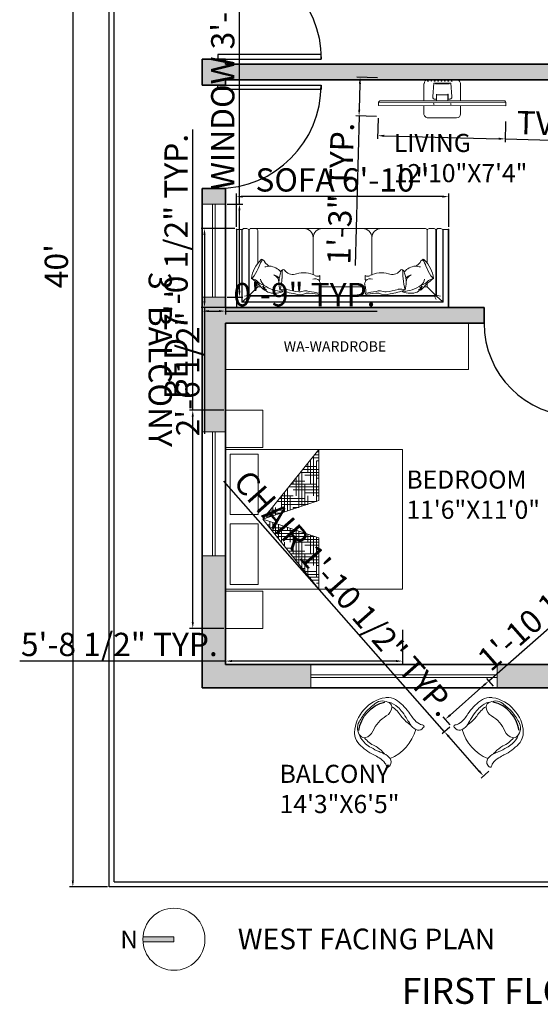
# Model space of a CAD drawing. Units: inches. Extents: x 2831 to 4250, y 1103 to 1797.
# Tile 1 of 15: x 3409 to 3610, y 1197 to 1578. Entities that reach past the tile are written whole.
import ezdxf

# ---------------------------------------------------------------- set-up
doc = ezdxf.new("R2010")
doc.units = ezdxf.units.IN
for name, color, linetype, lineweight in [('A-ANNO-DIMS', 2, 'Continuous', 18), ('A-ANNO-SYMB', 7, 'Continuous', 18), ('A-ANNO-TEXT', 7, 'Continuous', 18), ('A-ANNO-TITL', 7, 'Continuous', 25), ('A-AREA-IDEN', 7, 'Continuous', 18), ('A-DOOR', 4, 'Continuous', 25), ('A-EQPM', 8, 'Continuous', 18), ('A-FLOR-CASE', 9, 'Continuous', 18), ('A-WALL', 7, 'Continuous', 35), ('A-WALL-PATT', 252, 'Continuous', 13), ('C-PROP', 7, 'Continuous', 25), ('furn', 8, 'Continuous', 18), ('window', 130, 'Continuous', 18)]:
    doc.layers.add(name, color=color, linetype=linetype, lineweight=lineweight)
doc.layers.add('IFF-FURN-DETAIL', color=250, linetype='Continuous')
doc.styles.get("Standard").update_dxf_attribs({"font": 'arial.ttf'})
doc.dimstyles.new('ISO-25', dxfattribs={"dimtxt": 9, "dimasz": 2.5, "dimexe": 1.25, "dimexo": 0.625, "dimtad": 1, "dimdec": 1, "dimlunit": 3, "dimtxsty": 'Standard', "dimcen": 2.5, "dimadec": 0, "dimazin": 0, "dimtfac": 1, "dimtdec": 1, "dimtmove": 0, "dimatfit": 3, "dimfxl": 1, "dimarcsym": 0})

# ---------------------------------------------------------------- blocks, each defined once
blk = doc.blocks.new('*U2')
for p, q in [((0, 0), (0, -6)), ((40, 0), (40, -6))]:
    blk.add_line(p, q)
blk.add_lwpolyline([(0, 0), (0, 40), (1.75, 40), (1.75, 0)], close=True)
blk.add_arc((0, 0), 40, 0, 90)
blk = doc.blocks.new('*U3')
for p, q in [((0, 0), (0, -6)), ((36, 0), (36, -6))]:
    blk.add_line(p, q)
blk.add_lwpolyline([(0, 0), (0, 36), (1.75, 36), (1.75, 0)], close=True)
blk.add_arc((0, 0), 36, 0, 90)
blk = doc.blocks.new('*D6')
at = {"layer": 'A-ANNO-DIMS', "color": 0, "lineweight": -2, "transparency": 16777216}
for p, q in [((3442.6, 1722.51), (3427.96, 1722.51)), ((3429.21, 1720.01), (3429.21, 1245.01)), ((3442.6, 1242.51), (3427.96, 1242.51))]:
    blk.add_line(p, q, dxfattribs=at)
at = {"layer": 'A-ANNO-DIMS', "color": 0, "transparency": 16777216}
for points in [[(3428.79, 1720.01), (3429.62, 1720.01), (3429.21, 1722.51)], [(3428.79, 1245.01), (3429.62, 1245.01), (3429.21, 1242.51)]]:
    blk.add_solid(points, dxfattribs=at)
at = {"layer": 'Defpoints', "color": 0, "transparency": 16777216}
for p in [(3443.23, 1722.51), (3429.21, 1242.51), (3443.23, 1242.51)]:
    blk.add_point(p, dxfattribs=at)
at = {"layer": 'A-ANNO-DIMS', "color": 0, "transparency": 16777216, "insert": (3423.99, 1482.51), "char_height": 9, "attachment_point": 5, "rotation": 90}
blk.add_mtext("40'", dxfattribs=at)
blk = doc.blocks.new('COUCH6')
at = {"layer": 'furn'}
for p, q in [((-1.15, -0.846), (-1.15, 0)), ((-1.15, 0), (0, 0)), ((1.15, 0), (0, 0)), ((1.15, -0.846), (1.15, 0)), ((-1.145, -0.846), (-1.145, -0.005)), ((-1.145, -0.005), (0, -0.005)), ((-1.091, -0.845), (-1.091, -0.058)), ((-1.091, -0.058), (0, -0.058)), ((-1.086, -0.835), (-1.086, -0.063)), ((-1.086, -0.063), (0, -0.063)), ((-1.016, -0.124), (-1.086, -0.063)), ((-1.001, -0.114), (-1.014, -0.087)), ((1.145, -0.005), (0, -0.005)), ((1.091, -0.058), (0, -0.058)), ((1.086, -0.063), (0, -0.063)), ((1.001, -0.114), (1.014, -0.087)), ((1.016, -0.124), (1.086, -0.063)), ((1.086, -0.835), (1.086, -0.063)), ((1.091, -0.845), (1.091, -0.058)), ((1.145, -0.846), (1.145, -0.005)), ((-1.026, -0.131), (-1.061, -0.121)), ((-1.016, -0.835), (-1.016, -0.124)), ((-1.016, -0.124), (0, -0.124)), ((-1.011, -0.835), (-1.011, -0.129)), ((-1.011, -0.129), (0, -0.129)), ((-0.917, -0.223), (-1.011, -0.129)), ((-0.651, -0.171), (-0.652, -0.18)), ((1.016, -0.124), (0, -0.124)), ((1.011, -0.129), (0, -0.129)), ((0.651, -0.171), (0.652, -0.18)), ((0.917, -0.223), (1.011, -0.129)), ((1.011, -0.835), (1.011, -0.129)), ((1.016, -0.835), (1.016, -0.124)), ((1.026, -0.131), (1.061, -0.121)), ((-0.917, -0.223), (-0.884, -0.223)), ((-0.917, -0.259), (-0.917, -0.223)), ((-0.247, -0.223), (0, -0.223)), ((0.247, -0.223), (0, -0.223)), ((0.917, -0.223), (0.884, -0.223)), ((0.917, -0.259), (0.917, -0.223)), ((-0.665, -0.398), (-0.674, -0.359)), ((-0.651, -0.409), (-0.665, -0.398)), ((-0.318, -0.755), (-0.318, -0.351)), ((0.318, -0.755), (0.318, -0.355)), ((0.651, -0.409), (0.665, -0.398)), ((0.665, -0.398), (0.674, -0.359)), ((-0.917, -0.835), (-0.917, -0.48)), ((0.917, -0.835), (0.917, -0.48)), ((-1.145, -0.846), (-1.092, -0.846)), ((-1.091, -0.835), (-1.091, -0.845)), ((-1.091, -0.835), (-1.086, -0.835)), ((1.091, -0.835), (1.086, -0.835)), ((1.091, -0.835), (1.091, -0.845)), ((1.145, -0.846), (1.092, -0.846)), ((-1.036, -0.855), (-1.066, -0.855)), ((-0.937, -0.855), (-0.991, -0.855)), ((-0.418, -0.855), (-0.897, -0.855)), ((-0.218, -0.855), (-0.418, -0.855)), ((-0.218, -0.855), (0, -0.855)), ((0.218, -0.855), (0, -0.855)), ((0.218, -0.855), (0.418, -0.855)), ((0.418, -0.855), (0.991, -0.855)), ((0.937, -0.855), (0.991, -0.855)), ((0.937, -0.855), (0.991, -0.855)), ((1.036, -0.855), (1.066, -0.855))]:
    blk.add_line(p, q, dxfattribs=at)
for centre, radius, start, end in [((-0.693, -0.4), 0.26, 116.6172, 144.5701), ((-0.823, -0.23), 0.0392, 84.9285, 182.6706), ((-0.809, -0.237), 0.0473, 102.3256, 174.6372), ((-0.817, -0.249), 0.0419, 116.1434, 157.6281), ((-0.62, -0.58), 0.41, 94.3064, 124.2477), ((-0.735, -0.372), 0.218, 67.2195, 110.1562), ((-0.413, -0.269), 0.276, 163.2257, 199.1239), ((-0.39, -0.966), 0.828, 98.6756, 110.298), ((-1.233, -0.351), 0.578, 3.574, 16.2729), ((-0.625, -0.051), 0.148, 249.3987, 278.6386), ((-0.435, -0.699), 0.53, 93.9495, 108.4916), ((-0.461, -0.298), 0.16, 64.4969, 109.7129), ((-0.464, -0.312), 0.141, 68.1204, 93.31), ((-0.402, -0.079), 0.103, 264.9535, 292.5618), ((-0.374, 0.408), 0.562, 268.1099, 280.9598), ((-0.494, 1.007), 1.187, 276.3584, 281.8164), ((-0.26, -0.152), 0.0104, 337.6541, 129.2107), ((0.352, -0.179), 0.604, 177.8171, 180.6773), ((0.492, -0.117), 0.747, 185.2545, 188.1234), ((-0.492, -0.117), 0.747, 351.8766, 354.7455), ((0.26, -0.152), 0.0104, 50.7893, 202.3459), ((-0.352, -0.179), 0.604, 359.3227, 2.1829), ((0.494, 1.007), 1.187, 258.1836, 263.6416), ((0.374, 0.408), 0.562, 259.0402, 271.8901), ((0.402, -0.079), 0.103, 247.4382, 275.0465), ((0.461, -0.298), 0.16, 70.2871, 115.5031), ((0.464, -0.312), 0.141, 86.69, 111.8796), ((0.435, -0.699), 0.53, 71.5084, 86.0505), ((0.39, -0.966), 0.828, 69.702, 81.3244), ((0.625, -0.051), 0.148, 261.3614, 290.6013), ((0.735, -0.372), 0.218, 69.8438, 112.7805), ((0.62, -0.58), 0.41, 55.7523, 85.6936), ((1.233, -0.351), 0.578, 163.7271, 176.426), ((0.413, -0.269), 0.276, 340.8761, 16.7743), ((0.693, -0.4), 0.26, 35.4299, 63.3828), ((0.809, -0.237), 0.0473, 5.3628, 77.6744), ((0.823, -0.23), 0.0392, 357.3294, 95.0715), ((0.817, -0.249), 0.0419, 22.3719, 63.8566), ((-1.737, 0.688), 1.253, 306.9034, 311.5758), ((-1.136, 0.169), 0.506, 287.3558, 293.9344), ((-1.047, -0.4), 0.106, 32.1761, 54.0524), ((-0.663, -0.279), 0.324, 186.1069, 226.962), ((-0.809, -0.392), 0.157, 105.5409, 140.9927), ((-0.776, -0.327), 0.114, 130.9093, 169.8383), ((-0.778, -0.27), 0.0893, 293.1794, 356.9187), ((-0.759, -0.268), 0.0857, 280.6079, 328.6478), ((0.513, -0.305), 1.168, 180.4986, 185.1066), ((-0.296, -0.247), 0.0649, 245.5072, 314.4258), ((-0.231, -0.291), 0.0196, 155.4846, 217.9173), ((-0.332, -0.24), 0.0937, 332.6916, 351.8635), ((-0.307, -0.254), 0.0672, 0.1952, 27.3777), ((-0.406, -0.326), 0.161, 352.8843, 8.1753), ((0.307, -0.254), 0.0672, 152.6223, 179.8048), ((0.332, -0.24), 0.0937, 188.1365, 207.3084), ((0.406, -0.326), 0.161, 171.8247, 187.1157), ((0.231, -0.291), 0.0196, 322.0827, 24.5154), ((0.296, -0.247), 0.0649, 225.5742, 294.4928), ((-0.513, -0.305), 1.168, 354.8934, 359.5014), ((0.759, -0.268), 0.0857, 211.3522, 259.3921), ((0.778, -0.27), 0.0893, 183.0813, 246.8206), ((0.776, -0.327), 0.114, 10.1617, 49.0907), ((0.809, -0.392), 0.157, 39.0073, 74.4591), ((0.663, -0.279), 0.324, 313.038, 353.8931), ((1.737, 0.688), 1.253, 228.4242, 233.0966), ((1.136, 0.169), 0.506, 246.0656, 252.6442), ((1.047, -0.4), 0.106, 125.9476, 147.8239), ((-1.57, -0.729), 0.724, 22.8919, 32.1857), ((-0.813, -0.253), 0.197, 276.7688, 317.6018), ((-0.643, -0.386), 0.0242, 251.7544, 345.5556), ((-0.537, -0.477), 0.119, 70.4821, 134.6079), ((-0.421, -0.116), 0.261, 252.9517, 298.5304), ((-0.272, -0.389), 0.0505, 58.5546, 117.8039), ((0.272, -0.389), 0.0505, 62.1961, 121.4454), ((0.421, -0.116), 0.261, 241.4696, 287.0483), ((0.537, -0.477), 0.119, 45.3921, 109.5179), ((0.643, -0.386), 0.0242, 194.4444, 288.2456), ((0.813, -0.253), 0.197, 222.3982, 263.2312), ((1.57, -0.729), 0.724, 147.8143, 157.1081), ((-0.755, -0.41), 0.153, 194.1802, 223.196), ((-0.875, -0.514), 0.00886, 194.0721, 357.9619), ((-0.876, -0.478), 0.038, 284.8316, 343.5255), ((-0.767, -0.122), 0.326, 256.4531, 265.9689), ((-0.722, -0.582), 0.151, 116.9428, 141.4794), ((0.767, -0.122), 0.326, 274.0311, 283.5469), ((0.722, -0.582), 0.151, 38.5206, 63.0572), ((0.876, -0.478), 0.038, 196.4745, 255.1684), ((0.755, -0.41), 0.153, 316.804, 345.8198), ((0.875, -0.514), 0.00886, 182.0381, 345.9279), ((-1.148, -0.846), 0.0025, 180, 0), ((-1.092, -0.845), 0.001, 270, 0), ((-1.092, -0.845), 0.001, 270, 0), ((-1.092, -0.845), 0.001, 270, 0), ((-1.066, -0.835), 0.02, 180, 270), ((-1.036, -0.835), 0.02, 270, 0), ((-1.014, -0.835), 0.0025, 180, 0), ((-0.991, -0.835), 0.02, 180, 270), ((-0.937, -0.835), 0.02, 270, 360), ((-0.897, -0.835), 0.02, 180, 270), ((-0.418, -0.755), 0.1, 270, 0), ((-0.218, -0.755), 0.1, 180, 270), ((0.218, -0.755), 0.1, 270, 0), ((0.418, -0.755), 0.1, 180, 270), ((0.937, -0.835), 0.02, 180, 270), ((0.991, -0.835), 0.02, 270, 0), ((1.014, -0.835), 0.0025, 180, 0), ((1.036, -0.835), 0.02, 180, 270), ((1.066, -0.835), 0.02, 270, 0), ((1.092, -0.845), 0.001, 180, 270), ((1.092, -0.845), 0.001, 180, 270), ((1.092, -0.845), 0.001, 180, 270), ((1.148, -0.846), 0.0025, 180, 0)]:
    blk.add_arc(centre, radius, start, end, dxfattribs=at)
blk = doc.blocks.new('*X18')
at = {"color": 0}
for p, q in [((20.25, 14.812), (20.277, 14.812)), ((20.124, 14.688), (20.25, 14.688)), ((20.125, 14.5), (20.125, 14.689)), ((20.149, 14.719), (20.277, 14.719)), ((20.156, 14.625), (20.156, 14.728)), ((20.174, 14.75), (20.277, 14.75)), ((20.188, 14.75), (20.188, 14.767)), ((20.199, 14.781), (20.277, 14.781)), ((20.25, 14.319), (20.25, 14.75)), ((20.062, 14.257), (20.062, 14.612)), ((20.094, 14.375), (20.094, 14.65)), ((20.098, 14.656), (20.125, 14.656)), ((20.125, 14.594), (20.277, 14.594)), ((20.219, 14.309), (20.219, 14.625)), ((20.25, 14.625), (20.277, 14.625)), ((19.973, 14.5), (20.25, 14.5)), ((19.998, 14.531), (20.277, 14.531)), ((20, 14.237), (20, 14.5)), ((20.023, 14.562), (20.277, 14.562)), ((20.031, 14.247), (20.031, 14.573)), ((20.188, 14.299), (20.188, 14.5)), ((19.875, 14.25), (19.875, 14.379)), ((19.906, 14.375), (19.906, 14.417)), ((19.922, 14.438), (20, 14.438)), ((19.948, 14.469), (20.125, 14.469)), ((19.969, 14.226), (19.969, 14.375)), ((20, 14.375), (20.277, 14.375)), ((20.125, 14.406), (20.277, 14.406)), ((20.156, 14.288), (20.156, 14.375)), ((20.25, 14.438), (20.277, 14.438)), ((19.781, 14.164), (19.781, 14.262)), ((19.797, 14.281), (20.125, 14.281)), ((19.812, 14.174), (19.812, 14.301)), ((19.822, 14.312), (20.229, 14.312)), ((19.844, 14.185), (19.844, 14.34)), ((19.875, 14.344), (20.277, 14.344)), ((19.721, 14.188), (19.75, 14.188)), ((19.746, 14.219), (19.875, 14.219)), ((19.75, 14.154), (19.75, 14.223)), ((19.772, 14.25), (20, 14.25)), ((19.938, 14.216), (19.938, 14.25)), ((19.702, 14.094), (19.779, 14.094)), ((19.719, 14.073), (19.719, 14.114)), ((19.727, 14.062), (19.873, 14.062)), ((19.75, 14.034), (19.75, 14.103)), ((19.781, 13.995), (19.781, 14.093)), ((19.812, 14), (19.812, 14.082)), ((19.906, 13.84), (19.906, 14.051)), ((19.752, 14.031), (19.875, 14.031)), ((19.875, 13.878), (19.875, 14)), ((19.875, 13.969), (20.156, 13.969)), ((19.938, 13.801), (19.938, 14.041)), ((19.969, 13.875), (19.969, 14.031)), ((20, 14), (20, 14.02)), ((20, 14), (20.061, 14)), ((20.062, 13.645), (20.062, 14)), ((20.094, 13.625), (20.094, 13.989)), ((20.125, 13.75), (20.125, 13.979)), ((20.156, 13.875), (20.156, 13.969)), ((19.827, 13.938), (20.25, 13.938)), ((19.853, 13.906), (20.125, 13.906)), ((19.878, 13.875), (20, 13.875)), ((20.031, 13.684), (20.031, 13.875)), ((20.125, 13.844), (20.277, 13.844)), ((20.219, 13.451), (20.219, 13.875)), ((20.25, 13.5), (20.25, 13.937)), ((20.25, 13.875), (20.277, 13.875)), ((19.953, 13.781), (20.277, 13.781)), ((19.978, 13.75), (20.25, 13.75)), ((20, 13.812), (20.277, 13.812)), ((20, 13.723), (20, 13.75)), ((20.188, 13.49), (20.188, 13.75)), ((20.003, 13.719), (20.125, 13.719)), ((20.079, 13.625), (20.277, 13.625)), ((20.125, 13.656), (20.277, 13.656)), ((20.156, 13.529), (20.156, 13.625)), ((20.25, 13.688), (20.277, 13.688)), ((20.104, 13.594), (20.277, 13.594)), ((20.129, 13.562), (20.25, 13.562)), ((20.205, 13.469), (20.277, 13.469)), ((20.23, 13.438), (20.277, 13.438)), ((20.25, 13.5), (20.277, 13.5)), ((20.255, 13.406), (20.277, 13.406))]:
    blk.add_line(p, q, dxfattribs=at)
blk = doc.blocks.new('MAT-P02')
for p, q in [((-1.17, 0), (-1.17, -0.4)), ((-1.17, 0), (-0.77, 0)), ((-0.77, 0), (-0.77, -0.4)), ((-0.75, 0), (0.75, 0)), ((-0.75, 0), (-0.75, -1.9)), ((0.75, 0), (0.75, -1.9)), ((0.77, 0), (1.17, 0)), ((0.77, 0), (0.77, -0.4)), ((1.17, 0), (1.17, -0.4)), ((-0.7, -0.05), (-0.7, -0.35)), ((-0.7, -0.05), (-0.05, -0.05)), ((-0.05, -0.35), (-0.05, -0.05)), ((0.05, -0.05), (0.7, -0.05)), ((0.05, -0.35), (0.05, -0.05)), ((0.7, -0.05), (0.7, -0.35)), ((-1.17, -0.4), (-0.77, -0.4)), ((-0.75, -1.003), (0, -0.4)), ((0, -0.4), (-0.75, -1.003)), ((-0.7, -0.35), (-0.05, -0.35)), ((0, -0.4), (-0.2, -1.003)), ((0, -0.4), (0.2, -1.003)), ((0, -0.4), (0.75, -1.003)), ((0.05, -0.35), (0.7, -0.35)), ((0.77, -0.4), (1.17, -0.4)), ((-0.75, -1.003), (-0.2, -1.003)), ((0.2, -1.003), (0.75, -1.003)), ((0.75, -1.9), (-0.75, -1.9))]:
    blk.add_line(p, q)
at = {"xscale": -1, "rotation": 90}
blk.add_blockref('*X18', (14.128, 19.274), dxfattribs=at)
blk = doc.blocks.new('ILNG95')
for points in [[(120, 308, -0.32971), (51, 384, -0.036099), (50, 422, -0.497733), (75, 439, -0.070621), (96, 429, 0.101868), (133, 414, 0.091794), (259, 412, 0.024114), (351, 433, -0.090294), (638, 458, -0.132412), (775, 407, -0.068618), (816, 368, -0.184346), (943, 0, 1.803905)], [(120, 308, 0.138132), (244, 313, 0.001085), (325, 339, -0.034227), (462, 375, -0.033255), (567, 387, -0.137428), (727, 350, -4.561553)], [(120, 308, 0.138132), (244, 313, 0.001085), (325, 339, -0.034227), (462, 375, -0.033255), (567, 387, -0.137428), (727, 350, -4.561553)], [(235, 308, 0.064243), (394, 307, 0.04414), (433, 315, -0.118032), (643, 329, -6.296816)], [(235, 308, 0.064243), (394, 307, 0.04414), (433, 315, -0.118032), (643, 329, -6.296816)], [(639, 0, 0.078302), (612, 161, -0.233633), (633, 315, -0.28763), (710, 349, -0.317923), (875, 193, -0.032882), (900, 0, 1.140397)], [(639, 0, 0.078302), (612, 161, -0.233633), (633, 315, -0.28763), (710, 349, -0.317923), (875, 193, -0.032882), (900, 0, 1.140397)], [(120, -308, 0.32971), (51, -384, 0.036099), (50, -422, 0.497733), (75, -439, 0.070621), (96, -429, -0.101868), (133, -414, -0.091794), (259, -412, -0.024114), (351, -433, 0.090294), (638, -458, 0.132412), (775, -407, 0.068618), (816, -368, 0.184346), (943, 0, -1.803905)], [(639, 0, -0.078302), (612, -161, 0.233633), (633, -315, 0.28763), (710, -349, 0.317923), (875, -193, 0.032882), (900, 0, -1.140397)], [(639, 0, -0.078302), (612, -161, 0.233633), (633, -315, 0.28763), (710, -349, 0.317923), (875, -193, 0.032882), (900, 0, -1.140397)], [(120, -308, -0.138132), (244, -313, -0.001085), (325, -339, 0.034227), (462, -375, 0.033255), (567, -387, 0.137428), (727, -350, 4.561553)], [(120, -308, -0.138132), (244, -313, -0.001085), (325, -339, 0.034227), (462, -375, 0.033255), (567, -387, 0.137428), (727, -350, 4.561553)], [(235, -308, -0.064243), (394, -307, -0.04414), (433, -315, 0.118032), (643, -329, 6.296816)], [(235, -308, -0.064243), (394, -307, -0.04414), (433, -315, 0.118032), (643, -329, 6.296816)]]:
    blk.add_lwpolyline(points, format="xyb")
blk.add_arc((759, 1), 709, 154.3281, 205.801)
at = {"layer": 'IFF-FURN-DETAIL'}
blk.add_arc((326, -2), 549, 326.8997, 34.6691, dxfattribs=at)
blk.add_arc((326, -2), 549, 326.8997, 34.6691, dxfattribs=at)
blk = doc.blocks.new('TV')
at = {"color": 0}
for p, q in [((3967.27, 1784.85), (3967.05, 1784.65)), ((3967.76, 1763.68), (3967.54, 1763.86))]:
    blk.add_line(p, q, dxfattribs=at)
at = {"layer": 'window'}
for p, q in [((3967.54, 1763.86), (3967.05, 1784.65)), ((3964.41, 1777.23), (3967.22, 1777.3)), ((3968.01, 1777.32), (3969.36, 1777.35)), ((3966.53, 1775.82), (3964.33, 1775.61)), ((3964.34, 1775.34), (3964.45, 1775.34)), ((3964.34, 1775.31), (3964.43, 1775.32)), ((3966.14, 1775.2), (3967.01, 1775.22)), ((3966.14, 1775.18), (3967.27, 1775.2)), ((3966.14, 1775.18), (3966.14, 1775.2)), ((3966.3, 1773.29), (3966.26, 1775.18)), ((3964.39, 1773.06), (3964.48, 1773.06)), ((3964.39, 1773.04), (3964.5, 1773.04)), ((3966.61, 1772.66), (3964.4, 1772.77)), ((3966.19, 1773.28), (3967.31, 1773.31)), ((3966.19, 1773.26), (3967.05, 1773.28)), ((3966.19, 1773.26), (3966.19, 1773.28)), ((3964.55, 1771.15), (3967.36, 1771.22)), ((3968.15, 1771.24), (3969.5, 1771.27))]:
    blk.add_line(p, q, dxfattribs=at)
for points in [[(3968.33, 1763.69), (3967.83, 1784.86), (3967.27, 1784.85), (3967.76, 1763.68), (3968.33, 1763.69)], [(3963.86, 1771.81), (3963.75, 1776.54)], [(3970.16, 1771.96), (3970.05, 1776.69)], [(3964.4, 1772.77), (3964.33, 1775.61)], [(3964.48, 1773.06), (3964.43, 1775.32)], [(3964.5, 1773.04), (3964.45, 1775.34)]]:
    blk.add_lwpolyline(points, dxfattribs=at)
for points in [[(3966.53, 1775.82, -0.263666), (3966.93, 1775.69), (3967, 1775.57), (3967.01, 1775.22)], [(3966.61, 1772.66, 0.263666), (3967, 1772.81), (3967.06, 1772.93), (3967.05, 1773.28)]]:
    blk.add_lwpolyline(points, format="xyb", dxfattribs=at)
for centre, radius in [((3963.91, 1775.73), 0.0679), ((3963.93, 1775.17), 0.0679), ((3963.94, 1774.6), 0.0679), ((3967.77, 1775.68), 0.0451), ((3963.95, 1774.04), 0.0679), ((3963.97, 1773.48), 0.0679), ((3963.98, 1772.92), 0.0679), ((3967.83, 1772.86), 0.0451), ((3963.99, 1772.35), 0.0679), ((3964.01, 1771.79), 0.0679)]:
    blk.add_circle(centre, radius, dxfattribs=at)
for centre, start, end in [((3964.42, 1776.56), 91.3414, 181.3414), ((3969.38, 1776.67), 1.3414, 91.3414), ((3964.53, 1771.83), 181.3414, 271.3414), ((3969.49, 1771.94), 271.3414, 1.3414)]:
    blk.add_arc(centre, 0.676, start, end, dxfattribs=at)
blk = doc.blocks.new('WIN-36IN')
for p, q in [((0, 36), (9, 36)), ((4, 0), (4, 36)), ((5, 0), (5, 36)), ((0, 0), (9, 0))]:
    blk.add_line(p, q)
blk = doc.blocks.new('WIN-48IN')
for p, q in [((9, 48), (0, 48)), ((4, 0), (4, 48)), ((5, 0), (5, 48)), ((9, 0), (0, 0))]:
    blk.add_line(p, q)
blk = doc.blocks.new('WIN-72IN')
for p, q in [((0, 0), (0, 9)), ((72, 0), (72, 9)), ((0, 5), (72, 5)), ((0, 4), (72, 4))]:
    blk.add_line(p, q)
blk = doc.blocks.new('NORTH-MARK')
at = {"transparency": 33554687}
h = blk.add_hatch(color=256, dxfattribs=at)
h.dxf.hatch_style = 1
h.paths.add_polyline_path([(20.74, 13), (20.74, 11), (8.78, 11, -0.020861), (8.74, 12, -0.020861), (8.78, 13)])
for p, q in [((20.74, 13), (8.78, 13)), ((20.74, 11), (20.74, 13)), ((8.74, 11), (20.74, 11))]:
    blk.add_line(p, q)
blk.add_circle((20.74, 12), 12)
blk.add_text('N', height=6.9).set_placement((0, 8.47))
blk = doc.blocks.new('*D75')
at = {"layer": 'A-ANNO-DIMS', "color": 0, "lineweight": -2, "transparency": 16777216}
for p, q in [((3493.63, 1506.51), (3493.63, 1624.15)), ((3488.85, 1506.51), (3494.88, 1506.51)), ((3493.63, 1473.01), (3493.63, 1504.01)), ((3488.85, 1470.51), (3494.88, 1470.51))]:
    blk.add_line(p, q, dxfattribs=at)
at = {"layer": 'A-ANNO-DIMS', "color": 0, "transparency": 16777216}
for points in [[(3493.21, 1504.01), (3494.04, 1504.01), (3493.63, 1506.51)], [(3493.21, 1473.01), (3494.04, 1473.01), (3493.63, 1470.51)]]:
    blk.add_solid(points, dxfattribs=at)
at = {"layer": 'Defpoints', "color": 0, "transparency": 16777216}
for p in [(3488.23, 1506.51), (3493.63, 1506.51), (3488.23, 1470.51)]:
    blk.add_point(p, dxfattribs=at)
at = {"layer": 'A-ANNO-DIMS', "color": 0, "transparency": 16777216, "insert": (3488.34, 1566.58), "char_height": 9, "attachment_point": 5, "rotation": 90}
blk.add_mtext('WINDOW 3\'-0" TYP.', dxfattribs=at)
blk = doc.blocks.new('*D76')
at = {"layer": 'A-ANNO-DIMS', "color": 0, "lineweight": -2, "transparency": 16777216}
for p, q in [((3479.23, 1469.89), (3479.23, 1463.86)), ((3488.23, 1469.89), (3488.23, 1463.86)), ((3481.73, 1465.11), (3485.73, 1465.11)), ((3488.23, 1465.11), (3546.84, 1465.11))]:
    blk.add_line(p, q, dxfattribs=at)
at = {"layer": 'A-ANNO-DIMS', "color": 0, "transparency": 16777216}
for points in [[(3481.73, 1465.53), (3481.73, 1464.7), (3479.23, 1465.11)], [(3485.73, 1465.53), (3485.73, 1464.7), (3488.23, 1465.11)]]:
    blk.add_solid(points, dxfattribs=at)
at = {"layer": 'Defpoints', "color": 0, "transparency": 16777216}
for p in [(3479.23, 1470.51), (3488.23, 1470.51), (3488.23, 1465.11)]:
    blk.add_point(p, dxfattribs=at)
at = {"layer": 'A-ANNO-DIMS', "color": 0, "transparency": 16777216, "insert": (3518.78, 1470.33), "char_height": 9, "attachment_point": 5}
blk.add_mtext('0\'-9" TYP.', dxfattribs=at)
blk = doc.blocks.new('*D81')
at = {"layer": 'A-ANNO-DIMS', "color": 0, "lineweight": -2, "transparency": 16777216}
for p, q in [((3547.26, 1539.7), (3547.06, 1531.68)), ((3596.55, 1538.45), (3596.35, 1530.43)), ((3549.59, 1532.87), (3593.88, 1531.74)), ((3596.38, 1531.68), (3695.71, 1529.15))]:
    blk.add_line(p, q, dxfattribs=at)
at = {"layer": 'A-ANNO-DIMS', "color": 0, "transparency": 16777216}
for points in [[(3549.6, 1533.28), (3549.58, 1532.45), (3547.09, 1532.93)], [(3593.89, 1532.16), (3593.87, 1531.32), (3596.38, 1531.68)]]:
    blk.add_solid(points, dxfattribs=at)
at = {"layer": 'Defpoints', "color": 0, "transparency": 16777216}
for p in [(3547.28, 1540.32), (3596.57, 1539.07), (3596.38, 1531.68)]:
    blk.add_point(p, dxfattribs=at)
at = {"layer": 'A-ANNO-DIMS', "color": 0, "transparency": 16777216, "insert": (3647.43, 1535.66), "char_height": 9, "attachment_point": 5, "rotation": 358.5431}
blk.add_mtext('TV 4\'-1 1/2" TYP.', dxfattribs=at)
blk = doc.blocks.new('*D82')
at = {"layer": 'A-ANNO-DIMS', "color": 0, "lineweight": -2, "transparency": 16777216}
for p, q in [((3547.04, 1555.29), (3539.02, 1555.49)), ((3540.2, 1552.96), (3539.95, 1543.01)), ((3539.89, 1540.51), (3538.42, 1482.77)), ((3546.66, 1540.34), (3538.64, 1540.54))]:
    blk.add_line(p, q, dxfattribs=at)
at = {"layer": 'A-ANNO-DIMS', "color": 0, "transparency": 16777216}
for points in [[(3539.79, 1552.97), (3540.62, 1552.95), (3540.27, 1555.46)], [(3539.53, 1543.02), (3540.37, 1543), (3539.89, 1540.51)]]:
    blk.add_solid(points, dxfattribs=at)
at = {"layer": 'Defpoints', "color": 0, "transparency": 16777216}
for p in [(3547.66, 1555.27), (3539.89, 1540.51), (3547.28, 1540.32)]:
    blk.add_point(p, dxfattribs=at)
at = {"layer": 'A-ANNO-DIMS', "color": 0, "transparency": 16777216, "insert": (3533.9, 1510.52), "char_height": 9, "attachment_point": 5, "rotation": 88.5431}
blk.add_mtext('1\'-3" TYP.', dxfattribs=at)
blk = doc.blocks.new('*D83')
at = {"layer": 'A-ANNO-DIMS', "color": 0, "lineweight": -2, "transparency": 16777216}
for p, q in [((3475.58, 1426.81), (3475.58, 1535.34)), ((3487.6, 1426.81), (3474.33, 1426.81)), ((3475.58, 1344.98), (3475.58, 1424.31)), ((3487.6, 1342.48), (3474.33, 1342.48))]:
    blk.add_line(p, q, dxfattribs=at)
at = {"layer": 'A-ANNO-DIMS', "color": 0, "transparency": 16777216}
for points in [[(3475.16, 1424.31), (3475.99, 1424.31), (3475.58, 1426.81)], [(3475.16, 1344.98), (3475.99, 1344.98), (3475.58, 1342.48)]]:
    blk.add_solid(points, dxfattribs=at)
at = {"layer": 'Defpoints', "color": 0, "transparency": 16777216}
for p in [(3475.58, 1426.81), (3488.23, 1426.81), (3488.23, 1342.48)]:
    blk.add_point(p, dxfattribs=at)
at = {"layer": 'A-ANNO-DIMS', "color": 0, "transparency": 16777216, "insert": (3470.3, 1482.32), "char_height": 9, "attachment_point": 5, "rotation": 90}
blk.add_mtext('BED 7\'-0 1/2" TYP.', dxfattribs=at)
blk = doc.blocks.new('*D84')
at = {"layer": 'A-ANNO-DIMS', "color": 0, "lineweight": -2, "transparency": 16777216}
for p, q in [((3488.23, 1341.86), (3488.23, 1328.58)), ((3556.7, 1341.86), (3556.7, 1328.58)), ((3488.23, 1329.83), (3408.65, 1329.83)), ((3554.2, 1329.83), (3490.73, 1329.83))]:
    blk.add_line(p, q, dxfattribs=at)
at = {"layer": 'A-ANNO-DIMS', "color": 0, "transparency": 16777216}
for points in [[(3490.73, 1330.25), (3490.73, 1329.42), (3488.23, 1329.83)], [(3554.2, 1330.25), (3554.2, 1329.42), (3556.7, 1329.83)]]:
    blk.add_solid(points, dxfattribs=at)
at = {"layer": 'Defpoints', "color": 0, "transparency": 16777216}
for p in [(3488.23, 1342.48), (3556.7, 1342.48), (3488.23, 1329.83)]:
    blk.add_point(p, dxfattribs=at)
at = {"layer": 'A-ANNO-DIMS', "color": 0, "transparency": 16777216, "insert": (3447.19, 1335.11), "char_height": 9, "attachment_point": 5}
blk.add_mtext('5\'-8 1/2" TYP.', dxfattribs=at)
blk = doc.blocks.new('*D93')
at = {"layer": 'A-ANNO-DIMS', "color": 0, "lineweight": -2, "transparency": 16777216}
for p, q in [((3572.94, 1302.51), (3487.55, 1399.32)), ((3575.03, 1304.35), (3572, 1301.68)), ((3586.33, 1287.32), (3574.59, 1300.63)), ((3590.07, 1287.29), (3587.05, 1284.62))]:
    blk.add_line(p, q, dxfattribs=at)
at = {"layer": 'A-ANNO-DIMS', "color": 0, "transparency": 16777216}
for points in [[(3574.9, 1300.91), (3574.28, 1300.36), (3572.94, 1302.51)], [(3586.64, 1287.6), (3586.02, 1287.05), (3587.98, 1285.45)]]:
    blk.add_solid(points, dxfattribs=at)
at = {"layer": 'Defpoints', "color": 0, "transparency": 16777216}
for p in [(3572.94, 1302.51), (3575.5, 1304.76), (3590.54, 1287.7)]:
    blk.add_point(p, dxfattribs=at)
at = {"layer": 'A-ANNO-DIMS', "color": 0, "transparency": 16777216, "insert": (3533.38, 1355.34), "char_height": 9, "attachment_point": 5, "rotation": 311.4119}
blk.add_mtext('CHAIR 1\'-10 1/2" TYP.', dxfattribs=at)
blk = doc.blocks.new('*D94')
at = {"layer": 'A-ANNO-DIMS', "color": 0, "lineweight": -2, "transparency": 16777216}
for p, q in [((3590.07, 1322.17), (3654.36, 1378.87)), ((3591.91, 1320.08), (3589.24, 1323.11)), ((3575.11, 1308.98), (3588.2, 1320.52)), ((3575.08, 1305.23), (3572.41, 1308.26))]:
    blk.add_line(p, q, dxfattribs=at)
at = {"layer": 'A-ANNO-DIMS', "color": 0, "transparency": 16777216}
for points in [[(3587.92, 1320.83), (3588.47, 1320.2), (3590.07, 1322.17)], [(3574.84, 1309.29), (3575.39, 1308.66), (3573.24, 1307.32)]]:
    blk.add_solid(points, dxfattribs=at)
at = {"layer": 'Defpoints', "color": 0, "transparency": 16777216}
for p in [(3590.07, 1322.17), (3592.33, 1319.61), (3575.5, 1304.76)]:
    blk.add_point(p, dxfattribs=at)
at = {"layer": 'A-ANNO-DIMS', "color": 0, "transparency": 16777216, "insert": (3619.66, 1355.31), "char_height": 9, "attachment_point": 5, "rotation": 41.4119}
blk.add_mtext('1\'-10 1/2" TYP.', dxfattribs=at)
blk = doc.blocks.new('*D95')
at = {"layer": 'A-ANNO-DIMS', "color": 0, "lineweight": -2, "transparency": 16777216}
for p, q in [((3492.44, 1497.68), (3492.44, 1510.63)), ((3572.07, 1509.38), (3494.94, 1509.38)), ((3574.57, 1497.68), (3574.57, 1510.63))]:
    blk.add_line(p, q, dxfattribs=at)
at = {"layer": 'A-ANNO-DIMS', "color": 0, "transparency": 16777216}
for points in [[(3494.94, 1509.79), (3494.94, 1508.96), (3492.44, 1509.38)], [(3572.07, 1509.79), (3572.07, 1508.96), (3574.57, 1509.38)]]:
    blk.add_solid(points, dxfattribs=at)
at = {"layer": 'Defpoints', "color": 0, "transparency": 16777216}
for p in [(3492.44, 1509.38), (3492.44, 1497.06), (3574.57, 1497.06)]:
    blk.add_point(p, dxfattribs=at)
at = {"layer": 'A-ANNO-DIMS', "color": 0, "transparency": 16777216, "insert": (3533.5, 1514.66), "char_height": 9, "attachment_point": 5}
blk.add_mtext('SOFA 6\'-10"', dxfattribs=at)
blk = doc.blocks.new('*D96')
at = {"layer": 'A-ANNO-DIMS', "color": 0, "lineweight": -2, "transparency": 16777216}
for p, q in [((3491.81, 1497.06), (3478.87, 1497.06)), ((3480.12, 1494.56), (3480.12, 1469.01)), ((3491.81, 1466.51), (3478.87, 1466.51)), ((3480.12, 1466.51), (3480.12, 1417.71))]:
    blk.add_line(p, q, dxfattribs=at)
at = {"layer": 'A-ANNO-DIMS', "color": 0, "transparency": 16777216}
for points in [[(3479.7, 1494.56), (3480.53, 1494.56), (3480.12, 1497.06)], [(3479.7, 1469.01), (3480.53, 1469.01), (3480.12, 1466.51)]]:
    blk.add_solid(points, dxfattribs=at)
at = {"layer": 'Defpoints', "color": 0, "transparency": 16777216}
for p in [(3492.44, 1497.06), (3480.12, 1466.51), (3492.44, 1466.51)]:
    blk.add_point(p, dxfattribs=at)
at = {"layer": 'A-ANNO-DIMS', "color": 0, "transparency": 16777216, "insert": (3474.84, 1440.86), "char_height": 9, "attachment_point": 5, "rotation": 90}
blk.add_mtext('2\'-6 1/2"', dxfattribs=at)

msp = doc.modelspace()

# ---------------------------------------------------------------- hatches: boundary and pattern name
at = {"layer": 'A-WALL-PATT'}
h = msp.add_hatch(color=256, dxfattribs=at)
h.dxf.hatch_style = 1
h.paths.add_polyline_path([(3479.23, 1418.51), (3488.23, 1418.51), (3488.23, 1426.81), (3488.23, 1460.51), (3588.23, 1460.51), (3588.23, 1466.51), (3488.23, 1466.51), (3488.23, 1470.51), (3479.23, 1470.51)])
h.paths.add_polyline_path([(3488.23, 1506.51), (3488.23, 1512.51), (3479.23, 1512.51), (3479.23, 1506.51)])
h.paths.add_polyline_path([(3488.23, 1370.51), (3479.23, 1370.51), (3479.23, 1319.51), (3521.23, 1319.51), (3521.23, 1328.51), (3488.23, 1328.51)])
h.paths.add_polyline_path([(3794.23, 1319.51), (3794.23, 1247.51), (3614.23, 1247.51), (3614.23, 1242.51), (3803.23, 1242.51), (3803.23, 1328.51), (3767.23, 1328.51), (3767.23, 1394.51), (3758.23, 1394.51), (3758.23, 1328.51), (3635.23, 1328.51), (3635.23, 1460.51), (3637.23, 1460.51), (3637.23, 1466.51), (3624.23, 1466.51), (3624.23, 1460.51), (3626.23, 1460.51), (3626.23, 1328.51), (3593.23, 1328.51), (3593.23, 1319.51)])
h.paths.add_polyline_path([(3758.23, 1460.51), (3758.23, 1442.51), (3767.23, 1442.51), (3767.23, 1460.51), (3783.23, 1460.51), (3783.23, 1492.51), (3774.23, 1492.51), (3774.23, 1466.51), (3761.32, 1466.51), (3726.23, 1466.51), (3726.23, 1468.51), (3720.23, 1468.51), (3720.23, 1466.51), (3673.23, 1466.51), (3673.23, 1460.51)])
h.paths.add_polyline_path([(3597.63, 1698.24), (3687.22, 1698.24), (3687.22, 1717.46), (3597.63, 1717.46)], flags=9)
h.paths.add_polyline_path([(3776.75, 1438.29), (3776.75, 1360.77), (3795.97, 1360.77), (3795.97, 1438.29)], flags=25)
h.paths.add_polyline_path([(3453.37, 1482.95), (3453.37, 1401.85), (3472.59, 1401.85), (3472.59, 1482.95)], flags=9)
h.paths.add_polyline_path([(3506.21, 1267.1), (3560.71, 1267.1), (3560.71, 1293.71), (3506.21, 1293.71)], flags=9)
h.paths.add_polyline_path([(3760.5, 1579.7), (3798.74, 1579.7), (3798.74, 1602.51), (3760.5, 1602.51)], flags=9)
h.paths.add_polyline_path([(3617, 1637.95), (3659.12, 1637.95), (3659.12, 1660.76), (3617, 1660.76)], flags=9)
h.paths.add_polyline_path([(3679.39, 1612.63), (3728.46, 1612.63), (3728.46, 1639.25), (3679.39, 1639.25)], flags=9)
h.paths.add_polyline_path([(3731.07, 1499.72), (3773.19, 1499.72), (3773.19, 1522.53), (3731.07, 1522.53)], flags=9)
h.paths.add_polyline_path([(3652.82, 1496.49), (3701.95, 1496.49), (3701.95, 1523.1), (3652.82, 1523.1)], flags=9)
h.paths.add_polyline_path([(3550.37, 1510.97), (3604.5, 1510.97), (3604.5, 1537.58), (3550.37, 1537.58)], flags=9)
h.paths.add_polyline_path([(3514.45, 1612.63), (3570.67, 1612.63), (3570.67, 1639.25), (3514.45, 1639.25)], flags=9)
h = msp.add_hatch(color=256, dxfattribs=at)
h.dxf.hatch_style = 1
h.paths.add_polyline_path([(3783.23, 1560.51), (3767.23, 1560.51), (3767.23, 1572.51), (3761.23, 1572.51), (3758.23, 1572.51), (3758.23, 1560.51), (3488.23, 1560.51), (3488.23, 1562.51), (3485.23, 1562.51), (3479.23, 1562.51), (3479.23, 1552.51), (3485.23, 1552.51), (3488.23, 1552.51), (3488.23, 1554.51), (3642.23, 1554.51), (3642.23, 1498.51), (3648.23, 1498.51), (3648.23, 1554.51), (3720.23, 1554.51), (3720.23, 1498.51), (3726.23, 1498.51), (3726.23, 1554.51), (3774.23, 1554.51), (3774.23, 1528.51), (3783.23, 1528.51)])
h.paths.add_polyline_path([(3767.23, 1689.51), (3728.23, 1689.51), (3728.23, 1680.51), (3758.23, 1680.51), (3758.23, 1602.51), (3767.23, 1602.51)])
h.paths.add_polyline_path([(3680.23, 1689.51), (3656.23, 1689.51), (3656.23, 1680.51), (3662.23, 1680.51), (3662.23, 1608.51), (3644.23, 1608.51), (3644.23, 1602.51), (3668.23, 1602.51), (3668.23, 1680.51), (3680.23, 1680.51)])
h.paths.add_polyline_path([(3620.23, 1689.51), (3584.23, 1689.51), (3584.23, 1680.51), (3608.23, 1680.51), (3608.23, 1602.51), (3614.23, 1602.51), (3614.23, 1608.51), (3614.23, 1638.51), (3614.23, 1680.51), (3620.23, 1680.51)])
h.paths.add_polyline_path([(3512.23, 1689.51), (3479.23, 1689.51), (3479.23, 1665.51), (3488.23, 1665.51), (3488.23, 1680.51), (3512.23, 1680.51)])
h.paths.add_polyline_path([(3488.23, 1617.51), (3479.23, 1617.51), (3479.23, 1602.51), (3485.23, 1602.51), (3488.23, 1602.51)])

# ---------------------------------------------------------------- linework, layer by layer
at = {"layer": 'A-FLOR-CASE'}
for p, q in [((3582.23, 1442.51), (3582.23, 1460.51)), ((3488.23, 1442.51), (3582.23, 1442.51))]:
    msp.add_line(p, q, dxfattribs=at)
at = {"layer": 'A-WALL'}
for p, q in [((3479.23, 1562.51), (3488.23, 1562.51)), ((3479.23, 1552.51), (3479.23, 1562.51)), ((3488.23, 1560.51), (3488.23, 1562.51)), ((3488.23, 1560.51), (3758.23, 1560.51)), ((3488.23, 1554.51), (3642.23, 1554.51)), ((3488.23, 1552.51), (3488.23, 1554.51)), ((3479.23, 1552.51), (3488.23, 1552.51)), ((3479.23, 1319.51), (3479.23, 1512.51)), ((3479.23, 1512.51), (3488.23, 1512.51)), ((3488.23, 1466.51), (3488.23, 1512.51)), ((3488.23, 1466.51), (3588.23, 1466.51)), ((3588.23, 1460.51), (3588.23, 1466.51)), ((3488.23, 1328.51), (3488.23, 1460.51)), ((3488.23, 1460.51), (3588.23, 1460.51)), ((3488.23, 1328.51), (3626.23, 1328.51)), ((3479.23, 1319.51), (3794.23, 1319.51))]:
    msp.add_line(p, q, dxfattribs=at)
at = {"layer": 'C-PROP'}
msp.add_line((3445.23, 1244.51), (3614.23, 1244.51), dxfattribs=at)
msp.add_lwpolyline([(3443.23, 1722.51), (3803.23, 1722.51), (3803.23, 1242.51), (3443.23, 1242.51)], close=True, dxfattribs=at)
msp.add_lwpolyline([(3445.23, 1244.51), (3445.23, 1720.51), (3801.23, 1720.51)], dxfattribs=at)

# ---------------------------------------------------------------- block references
at = {"layer": 'A-ANNO-SYMB'}
msp.add_blockref('NORTH-MARK', (3447.56, 1210.3), dxfattribs=at)
at = {"layer": 'A-DOOR', "xscale": -1, "rotation": 270}
msp.add_blockref('*U2', (3485.23, 1562.51), dxfattribs=at)
at = {"layer": 'A-DOOR'}
for name, p, rotation in [('*U2', (3485.23, 1552.51), 270), ('*U3', (3624.23, 1460.51), 180)]:
    msp.add_blockref(name, p, dxfattribs=dict(at, rotation=rotation))
at = {"layer": 'A-EQPM', "xscale": 2.327319231123021, "yscale": 2.327319231123021, "zscale": 2.327319231123021, "rotation": 268.5430845181613}
msp.add_blockref('TV', (-321.11, 10881.54), dxfattribs=at)
at = {"layer": 'furn'}
for name, p, xscale, yscale, zscale, rotation in [('COUCH6', (3533.5, 1466.51), 35.70876312228397, 35.70876312228397, 35.70876312228397, 180), ('MAT-P02', (3488.23, 1384.65), 36.03633950593442, 36.03633950593442, 36.03633950593442, 90), ('ILNG95', (3559.02, 1295.81), -0.0243705291132055, 0.0243705291132055, 0.0243705291132055, 318.5881218623716), ('ILNG95', (3582.54, 1295.81), 0.0243705291132055, 0.0243705291132055, 0.0243705291132055, 41.41187813762839)]:
    msp.add_blockref(name, p, dxfattribs=dict(at, xscale=xscale, yscale=yscale, zscale=zscale, rotation=rotation))
at = {"layer": 'window'}
for name, p in [('WIN-36IN', (3479.23, 1470.51)), ('WIN-48IN', (3479.23, 1370.51))]:
    msp.add_blockref(name, p, dxfattribs=at)
at = {"layer": 'window', "rotation": 180}
msp.add_blockref('WIN-72IN', (3593.23, 1328.51), dxfattribs=at)

# ---------------------------------------------------------------- texts
at = {"layer": 'A-ANNO-TEXT', "insert": (3510.75, 1453.48), "char_height": 4, "attachment_point": 1}
msp.add_mtext_dynamic_manual_height_columns('WA-WARDROBE', width=29.5334, gutter_width=12.5, heights=[0], dxfattribs=at)
at = {"layer": 'A-ANNO-TITL', "attachment_point": 1}
for s, insert, char_height in [('{\\fTimes New Roman|b0|i0|c0|p18;WEST FACING PLAN}', (3492.99, 1226.42), 8), ('{\\fTimes New Roman|b0|i0|c0|p18;FIRST FLOOR PLAN}', (3556.39, 1207.34), 10)]:
    msp.add_mtext_dynamic_manual_height_columns(s, width=196.2607, gutter_width=12.5, heights=[0], dxfattribs=dict(at, insert=insert, char_height=char_height))
at = {"layer": 'A-AREA-IDEN', "char_height": 7, "attachment_point": 1}
for s, insert in [('{\\fTimes New Roman|b0|i0|c0|p18;LIVING\\P12\'10"X7\'4"}', (3553.33, 1533.62)), ('{\\fTimes New Roman|b0|i0|c0|p18;BEDROOM\\P11\'6"X11\'0"}', (3558.21, 1403.5)), ('{\\fTimes New Roman|b0|i0|c0|p18;BALCONY\\P14\'3"X6\'5"}', (3509.17, 1289.75))]:
    msp.add_mtext_dynamic_manual_height_columns(s, width=81.5075, gutter_width=12.5, heights=[0], dxfattribs=dict(at, insert=insert))
at = {"layer": 'A-AREA-IDEN', "insert": (3467.5, 1480.16), "char_height": 9, "attachment_point": 1, "rotation": 270}
msp.add_mtext_dynamic_manual_height_columns("{\\fTimes New Roman|b0|i0|c0|p18;3' BALCONY}", width=81.5075, gutter_width=12.5, heights=[0], dxfattribs=at)

# ---------------------------------------------------------------- dimensions: what is measured, and where the dimension line sits
at = {"layer": 'A-ANNO-DIMS'}
for base, p1, p2, angle, override, picture, middle in [((3429.21, 1242.51), (3443.23, 1722.51), (3443.23, 1242.51), 90, {"dimclrd": 0, "dimclre": 0, "dimclrt": 0}, '*D6', (3423.99, 1482.51)), ((3480.1171, 1466.5133), (3492.4374, 1497.0567), (3492.4374, 1466.5133), 270, {"dimdec": 1, "dimlfac": 1, "dimrnd": 0, "dimzin": 1, "dimdsep": 46, "dimlunit": 4, "dimfrac": 2}, '*D96', (3474.8387, 1440.8637))]:
    dim = msp.add_linear_dim(base=base, p1=p1, p2=p2, angle=angle, dimstyle='ISO-25', override=override, dxfattribs=at)
    dim.commit()
    dim.dimension.update_dxf_attribs({"geometry": picture, "text_midpoint": middle})
for base, p1, p2, angle, text, picture, middle in [((3493.63, 1506.51), (3488.23, 1470.51), (3488.23, 1506.51), 90, 'WINDOW <> TYP.', '*D75', (3488.34, 1566.58)), ((3596.38, 1531.68), (3547.28, 1540.32), (3596.57, 1539.07), 358.5431, 'TV <> TYP.', '*D81', (3647.43, 1535.66)), ((3539.89, 1540.51), (3547.66, 1555.27), (3547.28, 1540.32), 268.5431, '<> TYP.', '*D82', (3533.9, 1510.52)), ((3475.58, 1426.81), (3488.23, 1342.48), (3488.23, 1426.81), 90, 'BED <> TYP.', '*D83', (3470.3, 1482.32)), ((3492.44, 1509.38), (3574.57, 1497.06), (3492.44, 1497.06), 180, 'SOFA <>', '*D95', (3533.5, 1514.66)), ((3572.94, 1302.51), (3590.54, 1287.7), (3575.5, 1304.76), 131.4119, 'CHAIR <> TYP.', '*D93', (3533.38, 1355.34)), ((3590.07, 1322.17), (3575.5, 1304.76), (3592.33, 1319.61), 41.4119, '<> TYP.', '*D94', (3619.66, 1355.31)), ((3488.23, 1329.83), (3556.7, 1342.48), (3488.23, 1342.48), 180, '<> TYP.', '*D84', (3447.19, 1335.11))]:
    dim = msp.add_linear_dim(base=base, p1=p1, p2=p2, angle=angle, text=text, dimstyle='ISO-25', override={"dimdec": 1, "dimlfac": 1, "dimrnd": 0, "dimzin": 1, "dimdsep": 46, "dimlunit": 4, "dimfrac": 2}, dxfattribs=at)
    dim.commit()
    dim.dimension.update_dxf_attribs({"geometry": picture, "text_midpoint": middle})
dim = msp.add_linear_dim(base=(3488.23, 1465.11), p1=(3479.23, 1470.51), p2=(3488.23, 1470.51), text='<> TYP.', dimstyle='ISO-25', override={"dimdec": 1, "dimlfac": 1, "dimrnd": 0, "dimzin": 1, "dimdsep": 46, "dimlunit": 4, "dimfrac": 2}, dxfattribs=at)
dim.commit()
dim.dimension.update_dxf_attribs({"geometry": '*D76', "text_midpoint": (3518.78, 1470.33)})

doc.saveas('drawing.dxf')
